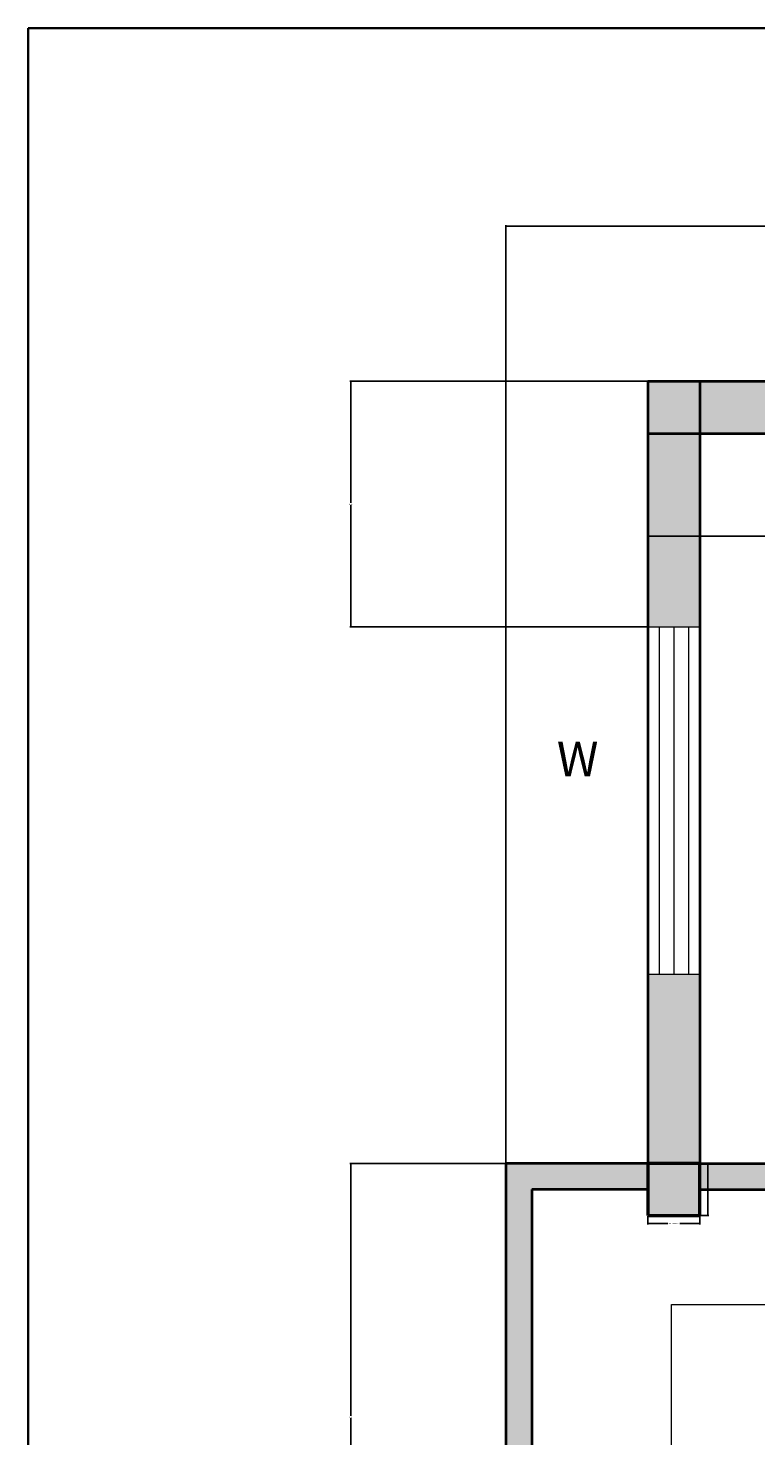
# Model space of a CAD drawing. Units: inches. Extents: x 25176543 to 25177243, y 80295576 to 80296086.
# Tile 2 of 11: x 25176543 to 25176668, y 80295843 to 80296086. Entities that reach past the tile are written whole.
import ezdxf

# ---------------------------------------------------------------- set-up
doc = ezdxf.new("R2010")
doc.units = ezdxf.units.IN
doc.header["$MEASUREMENT"] = 0
for name, color, linetype, lineweight in [('A-ANNO-DIMS', 2, 'Continuous', 18), ('A-ANNO-IDEN', 7, 'Continuous', 18), ('A-ANNO-SYMB', 7, 'Continuous', 18), ('A-ANNO-TTLB', 7, 'Continuous', 35), ('A-COLS', 7, 'Continuous', 50), ('A-COLS-PATT', 251, 'Continuous', 13), ('A-GLAZ', 4, 'Continuous', 18), ('A-WALL', 7, 'Continuous', 40), ('A-WALL-PATT', 146, 'Continuous', 13)]:
    doc.layers.add(name, color=color, linetype=linetype, lineweight=lineweight)
doc.styles.get("Standard").update_dxf_attribs({"font": 'arial.ttf'})
doc.dimstyles.get("Standard").update_dxf_attribs({"dimtxt": 0.18, "dimasz": 0.18, "dimexe": 0.18, "dimexo": 0.0625, "dimgap": 0.09, "dimtad": 0, "dimtih": 1, "dimtoh": 1, "dimdec": 4, "dimzin": 0, "dimdsep": 46, "dimtxsty": 'Standard', "dimcen": 0.09, "dimadec": 0, "dimazin": 0, "dimtfac": 1, "dimtdec": 4, "dimtofl": 0, "dimtmove": 0, "dimatfit": 3, "dimfxl": 1, "dimtolj": 1, "dimtzin": 0, "dimarcsym": 0})

# ---------------------------------------------------------------- blocks, each defined once
blk = doc.blocks.new('WIN-60IN')
for p, q in [((0, 9), (0, 0)), ((60, 9), (0, 9)), ((0, 9), (0, 4.5)), ((60, 0), (60, 9)), ((60, 7), (0, 7)), ((0, 4.5), (60, 4.5)), ((0, 2), (60, 2)), ((0, 0), (60, 0))]:
    blk.add_line(p, q)
blk = doc.blocks.new('COLUMN-9IN-SQ')
for p, q in [((9, 9), (0, 9)), ((0, 9), (0, 0)), ((9, 0), (9, 9)), ((0, 0), (9, 0))]:
    blk.add_line(p, q)
blk = doc.blocks.new('*D24')
at = {"layer": 'A-ANNO-DIMS', "color": 0, "lineweight": -2, "transparency": 16777216}
for p, q in [((25176649.8, 80295881.24), (25176649.8, 80295879.77)), ((25176649.98, 80295879.95), (25176653.26, 80295879.95)), ((25176658.62, 80295879.95), (25176655.34, 80295879.95)), ((25176658.8, 80295881.24), (25176658.8, 80295879.77))]:
    blk.add_line(p, q, dxfattribs=at)
at = {"layer": 'A-ANNO-DIMS', "color": 0, "transparency": 16777216}
for points in [[(25176649.98, 80295879.98), (25176649.98, 80295879.92), (25176649.8, 80295879.95)], [(25176658.62, 80295879.98), (25176658.62, 80295879.92), (25176658.8, 80295879.95)]]:
    blk.add_solid(points, dxfattribs=at)
at = {"layer": 'Defpoints', "color": 0, "transparency": 16777216}
for p in [(25176649.8, 80295881.3), (25176658.8, 80295881.3), (25176658.8, 80295879.95)]:
    blk.add_point(p, dxfattribs=at)
at = {"layer": 'A-ANNO-DIMS', "color": 0, "transparency": 16777216, "insert": (25176654.3, 80295879.95), "char_height": 0.18, "attachment_point": 5}
blk.add_mtext('\\A1;COLUMN 9 TYP.', dxfattribs=at)
blk = doc.blocks.new('*D25')
at = {"layer": 'A-ANNO-DIMS', "color": 0, "lineweight": -2, "transparency": 16777216}
for p, q in [((25176658.86, 80295890.3), (25176660.33, 80295890.3)), ((25176660.15, 80295890.12), (25176660.15, 80295885.98)), ((25176660.15, 80295881.48), (25176660.15, 80295885.62)), ((25176658.86, 80295881.3), (25176660.33, 80295881.3))]:
    blk.add_line(p, q, dxfattribs=at)
at = {"layer": 'A-ANNO-DIMS', "color": 0, "transparency": 16777216}
for points in [[(25176660.12, 80295890.12), (25176660.18, 80295890.12), (25176660.15, 80295890.3)], [(25176660.12, 80295881.48), (25176660.18, 80295881.48), (25176660.15, 80295881.3)]]:
    blk.add_solid(points, dxfattribs=at)
at = {"layer": 'Defpoints', "color": 0, "transparency": 16777216}
for p in [(25176658.8, 80295890.3), (25176660.15, 80295890.3), (25176658.8, 80295881.3)]:
    blk.add_point(p, dxfattribs=at)
at = {"layer": 'A-ANNO-DIMS', "color": 0, "transparency": 16777216, "insert": (25176660.15, 80295885.8), "char_height": 0.18, "attachment_point": 5}
blk.add_mtext('\\A1;9 TYP.', dxfattribs=at)
blk = doc.blocks.new('*D48')
at = {"layer": 'A-ANNO-DIMS', "color": 0, "lineweight": -2, "transparency": 16777216}
for p, q in [((25176625.3, 80295890.36), (25176625.3, 80296052.23)), ((25176625.48, 80296052.05), (25176875.16, 80296052.05)), ((25177125.62, 80296052.05), (25176875.95, 80296052.05)), ((25177125.8, 80296025.36), (25177125.8, 80296052.23))]:
    blk.add_line(p, q, dxfattribs=at)
at = {"layer": 'A-ANNO-DIMS', "color": 0, "transparency": 16777216}
for points in [[(25176625.48, 80296052.08), (25176625.48, 80296052.02), (25176625.3, 80296052.05)], [(25177125.62, 80296052.08), (25177125.62, 80296052.02), (25177125.8, 80296052.05)]]:
    blk.add_solid(points, dxfattribs=at)
at = {"layer": 'Defpoints', "color": 0, "transparency": 16777216}
for p in [(25177125.8, 80296052.05), (25177125.8, 80296025.3), (25176625.3, 80295890.3)]:
    blk.add_point(p, dxfattribs=at)
at = {"layer": 'A-ANNO-DIMS', "color": 0, "transparency": 16777216, "insert": (25176875.55, 80296052.05), "char_height": 0.18, "attachment_point": 5}
blk.add_mtext('\\A1;500.5', dxfattribs=at)
blk = doc.blocks.new('*D51')
at = {"layer": 'A-ANNO-DIMS', "color": 0, "lineweight": -2, "transparency": 16777216}
for p, q in [((25176625.24, 80295890.3), (25176598.37, 80295890.3)), ((25176598.55, 80295890.12), (25176598.55, 80295846.73)), ((25176598.55, 80295802.98), (25176598.55, 80295846.37)), ((25176625.24, 80295802.8), (25176598.37, 80295802.8))]:
    blk.add_line(p, q, dxfattribs=at)
at = {"layer": 'A-ANNO-DIMS', "color": 0, "transparency": 16777216}
for points in [[(25176598.52, 80295890.12), (25176598.58, 80295890.12), (25176598.55, 80295890.3)], [(25176598.52, 80295802.98), (25176598.58, 80295802.98), (25176598.55, 80295802.8)]]:
    blk.add_solid(points, dxfattribs=at)
at = {"layer": 'Defpoints', "color": 0, "transparency": 16777216}
for p in [(25176598.55, 80295890.3), (25176625.3, 80295890.3), (25176625.3, 80295802.8)]:
    blk.add_point(p, dxfattribs=at)
at = {"layer": 'A-ANNO-DIMS', "color": 0, "transparency": 16777216, "insert": (25176598.55, 80295846.55), "char_height": 0.18, "attachment_point": 5}
blk.add_mtext('\\A1;87.5', dxfattribs=at)
blk = doc.blocks.new('*D58')
at = {"layer": 'A-ANNO-DIMS', "color": 0, "lineweight": -2, "transparency": 16777216}
for p, q in [((25176649.74, 80296025.3), (25176598.37, 80296025.3)), ((25176598.55, 80296025.12), (25176598.55, 80296004.3)), ((25176598.55, 80295983.11), (25176598.55, 80296003.93)), ((25176649.74, 80295982.93), (25176598.37, 80295982.93))]:
    blk.add_line(p, q, dxfattribs=at)
at = {"layer": 'A-ANNO-DIMS', "color": 0, "transparency": 16777216}
for points in [[(25176598.52, 80296025.12), (25176598.58, 80296025.12), (25176598.55, 80296025.3)], [(25176598.52, 80295983.11), (25176598.58, 80295983.11), (25176598.55, 80295982.93)]]:
    blk.add_solid(points, dxfattribs=at)
at = {"layer": 'Defpoints', "color": 0, "transparency": 16777216}
for p in [(25176598.55, 80296025.3), (25176649.8, 80296025.3), (25176649.8, 80295982.93)]:
    blk.add_point(p, dxfattribs=at)
at = {"layer": 'A-ANNO-DIMS', "color": 0, "transparency": 16777216, "insert": (25176598.55, 80296004.11), "char_height": 0.18, "attachment_point": 5}
blk.add_mtext('\\A1;42.38', dxfattribs=at)
blk = doc.blocks.new('*D63')
at = {"layer": 'A-ANNO-DIMS', "color": 0, "lineweight": -2, "transparency": 16777216}
for p, q in [((25176649.8, 80296025.24), (25176649.8, 80295998.37)), ((25176695.19, 80296025.24), (25176695.19, 80295998.37)), ((25176649.98, 80295998.55), (25176672.1, 80295998.55)), ((25176695.01, 80295998.55), (25176672.89, 80295998.55))]:
    blk.add_line(p, q, dxfattribs=at)
at = {"layer": 'A-ANNO-DIMS', "color": 0, "transparency": 16777216}
for points in [[(25176649.98, 80295998.58), (25176649.98, 80295998.52), (25176649.8, 80295998.55)], [(25176695.01, 80295998.58), (25176695.01, 80295998.52), (25176695.19, 80295998.55)]]:
    blk.add_solid(points, dxfattribs=at)
at = {"layer": 'Defpoints', "color": 0, "transparency": 16777216}
for p in [(25176649.8, 80296025.3), (25176695.19, 80296025.3), (25176649.8, 80295998.55)]:
    blk.add_point(p, dxfattribs=at)
at = {"layer": 'A-ANNO-DIMS', "color": 0, "transparency": 16777216, "insert": (25176672.5, 80295998.55), "char_height": 0.18, "attachment_point": 5}
blk.add_mtext('\\A1;45.39', dxfattribs=at)

msp = doc.modelspace()

# ---------------------------------------------------------------- hatches: boundary and pattern name
at = {"layer": 'A-COLS-PATT'}
h = msp.add_hatch(color=256, dxfattribs=at)
h.dxf.hatch_style = 1
h.paths.add_polyline_path([(25176658.8016, 80296025.3022), (25176649.8016, 80296025.3022), (25176649.8016, 80296016.3022), (25176658.8016, 80296016.3022)])
h.paths.add_polyline_path([(25176819.3016, 80296025.3022), (25176810.3016, 80296025.3022), (25176810.3016, 80296016.3022), (25176819.3016, 80296016.3022)])
h.paths.add_polyline_path([(25176876.3016, 80296025.3022), (25176867.3016, 80296025.3022), (25176867.3016, 80296016.3022), (25176876.3016, 80296016.3022)])
h.paths.add_polyline_path([(25177013.3016, 80296025.3022), (25177004.3016, 80296025.3022), (25177004.3016, 80296016.3022), (25177013.3016, 80296016.3022)])
h.paths.add_polyline_path([(25176819.3016, 80295890.3022), (25176810.3016, 80295890.3022), (25176810.3016, 80295881.3022), (25176819.3016, 80295881.3022)])
h.paths.add_polyline_path([(25176658.8016, 80295890.3022), (25176649.8016, 80295890.3022), (25176649.8016, 80295881.3022), (25176658.8016, 80295881.3022)])
h.paths.add_polyline_path([(25177125.8016, 80296025.3022), (25177116.8016, 80296025.3022), (25177116.8016, 80296016.3022), (25177125.8016, 80296016.3022)])
h.paths.add_polyline_path([(25177125.8016, 80295848.3022), (25177116.8016, 80295848.3022), (25177116.8016, 80295839.3022), (25177125.8016, 80295839.3022)])
h.paths.add_polyline_path([(25177013.3016, 80295848.3022), (25177004.3016, 80295848.3022), (25177004.3016, 80295839.3022), (25177013.3016, 80295839.3022)])
h.paths.add_polyline_path([(25177125.8016, 80295676.8022), (25177116.8016, 80295676.8022), (25177116.8016, 80295667.8022), (25177125.8016, 80295667.8022)])
h.paths.add_polyline_path([(25177013.3016, 80295676.8022), (25177004.3016, 80295676.8022), (25177004.3016, 80295667.8022), (25177013.3016, 80295667.8022)])
h.paths.add_polyline_path([(25176842.3016, 80295676.8022), (25176833.3016, 80295676.8022), (25176833.3016, 80295667.8022), (25176842.3016, 80295667.8022)])
h.paths.add_polyline_path([(25176893.3016, 80295676.8022), (25176884.3016, 80295676.8022), (25176884.3016, 80295667.8022), (25176893.3016, 80295667.8022)])
h.paths.add_polyline_path([(25176842.3016, 80295807.3022), (25176833.3016, 80295807.3022), (25176833.3016, 80295798.3022), (25176842.3016, 80295798.3022)])
h.paths.add_polyline_path([(25176658.8016, 80295807.3022), (25176649.8016, 80295807.3022), (25176649.8016, 80295798.3022), (25176658.8016, 80295798.3022)])
h.paths.add_polyline_path([(25176658.8016, 80295676.8022), (25176649.8016, 80295676.8022), (25176649.8016, 80295667.8022), (25176658.8016, 80295667.8022)])
at = {"layer": 'A-WALL-PATT'}
h = msp.add_hatch(color=256, dxfattribs=at)
h.dxf.hatch_style = 1
h.paths.add_polyline_path([(25176695.189, 80296025.3022), (25176658.8016, 80296025.3022), (25176658.8016, 80296016.3022), (25176695.189, 80296016.3022)])
h.paths.add_polyline_path([(25176810.3016, 80296025.3022), (25176755.189, 80296025.3022), (25176755.189, 80296016.3022), (25176810.3016, 80296016.3022)])
h.paths.add_polyline_path([(25176819.3016, 80296016.3022), (25176814.8016, 80296016.3022), (25176814.8016, 80295965.3022), (25176819.3016, 80295965.3022)], flags=17)
h.paths.add_polyline_path([(25176828.0421, 80296025.3022), (25176819.3016, 80296025.3022), (25176819.3016, 80296016.3022), (25176828.0421, 80296016.3022)])
h.paths.add_polyline_path([(25176867.3016, 80296025.3022), (25176852.0421, 80296025.3022), (25176852.0421, 80296016.3022), (25176867.3016, 80296016.3022)])
h.paths.add_polyline_path([(25176885.1873, 80296025.3022), (25176876.3016, 80296025.3022), (25176876.3016, 80296016.3022), (25176885.1873, 80296016.3022)])
h.paths.add_polyline_path([(25176919.8016, 80296025.3022), (25176909.1873, 80296025.3022), (25176909.1873, 80296016.3022), (25176919.8016, 80296016.3022)])
h.paths.add_polyline_path([(25176924.3016, 80296016.3022), (25176919.8016, 80296016.3022), (25176919.8016, 80295890.3022), (25176904.8016, 80295890.3022), (25176904.8016, 80295885.8022), (25176967.3016, 80295885.8022), (25176967.3016, 80295890.3022), (25176924.3016, 80295890.3022)])
h.paths.add_polyline_path([(25176924.3016, 80296025.3022), (25176919.8016, 80296025.3022), (25176919.8016, 80296016.3022), (25176924.3016, 80296016.3022)])
h.paths.add_polyline_path([(25176938.7147, 80296025.3022), (25176924.3016, 80296025.3022), (25176924.3016, 80296016.3022), (25176938.7147, 80296016.3022)])
h.paths.add_polyline_path([(25176871.8016, 80296016.3022), (25176867.3016, 80296016.3022), (25176867.3016, 80295932.3022), (25176819.3016, 80295932.3022), (25176819.3016, 80295933.3022), (25176814.8016, 80295933.3022), (25176814.8016, 80295932.3022), (25176814.8016, 80295927.3022), (25176819.3016, 80295927.3022), (25176819.3016, 80295927.8022), (25176867.3016, 80295927.8022), (25176867.3016, 80295885.8022), (25176871.8016, 80295885.8022), (25176872.8016, 80295885.8022), (25176872.8016, 80295890.3022), (25176871.8016, 80295890.3022)])
h.paths.add_polyline_path([(25177004.3016, 80296025.3022), (25176986.7147, 80296025.3022), (25176986.7147, 80296016.3022), (25177004.3016, 80296016.3022)])
h.paths.add_polyline_path([(25177035.845, 80296025.3022), (25177013.3016, 80296025.3022), (25177013.3016, 80296016.3022), (25177035.845, 80296016.3022)])
h.paths.add_polyline_path([(25177008.8016, 80296016.3022), (25177004.3016, 80296016.3022), (25177004.3016, 80295890.3022), (25177003.3016, 80295890.3022), (25177003.3016, 80295885.8022), (25177004.3016, 80295885.8022), (25177004.3016, 80295885.3022), (25177008.8016, 80295885.3022)])
h.paths.add_polyline_path([(25177116.8016, 80296025.3022), (25177095.845, 80296025.3022), (25177095.845, 80296016.3022), (25177116.8016, 80296016.3022)])
h.paths.add_polyline_path([(25177125.8016, 80296016.3022), (25177116.8016, 80296016.3022), (25177116.8016, 80295971.1334), (25177121.3016, 80295971.1334), (25177125.8016, 80295971.1334)])
h.paths.add_polyline_path([(25177116.8016, 80295848.3022), (25177013.3016, 80295848.3022), (25177013.3016, 80295843.8022), (25177116.8016, 80295843.8022)])
h.paths.add_polyline_path([(25177125.8016, 80295911.1334), (25177116.8016, 80295911.1334), (25177116.8016, 80295848.3022), (25177125.8016, 80295848.3022)])
h.paths.add_polyline_path([(25177008.8016, 80295802.3022), (25177004.3016, 80295802.3022), (25177004.3016, 80295676.8022), (25177008.8016, 80295676.8022)])
h.paths.add_polyline_path([(25176658.8016, 80295705.5694), (25176649.8016, 80295705.5694), (25176649.8016, 80295676.8022), (25176658.8016, 80295676.8022)])
h.paths.add_polyline_path([(25176658.8016, 80295798.3022), (25176649.8016, 80295798.3022), (25176649.8016, 80295765.5694), (25176654.3016, 80295765.5694), (25176658.8016, 80295765.5694)])
h.paths.add_polyline_path([(25176833.3016, 80295807.3022), (25176658.8016, 80295807.3022), (25176658.8016, 80295802.8022), (25176833.3016, 80295802.8022)])
h.paths.add_polyline_path([(25176842.3016, 80295761.3022), (25176837.8016, 80295761.3022), (25176837.8016, 80295676.8022), (25176842.3016, 80295676.8022)])
h.paths.add_polyline_path([(25176649.8016, 80295807.3022), (25176629.8016, 80295807.3022), (25176629.8016, 80295885.8022), (25176649.8016, 80295885.8022), (25176649.8016, 80295890.3022), (25176625.3016, 80295890.3022), (25176625.3016, 80295802.8022), (25176649.8016, 80295802.8022)])
h.paths.add_polyline_path([(25176810.3016, 80295890.3022), (25176658.8016, 80295890.3022), (25176658.8016, 80295885.8022), (25176810.3016, 80295885.8022)])
h.paths.add_polyline_path([(25176658.8016, 80295922.9263), (25176649.8016, 80295922.9263), (25176649.8016, 80295890.3022), (25176658.8016, 80295890.3022)])
h.paths.add_polyline_path([(25176658.8016, 80296016.3022), (25176649.8016, 80296016.3022), (25176649.8016, 80295982.9263), (25176654.3016, 80295982.9263), (25176658.8016, 80295982.9263)])

# ---------------------------------------------------------------- linework, layer by layer
at = {"layer": 'A-ANNO-SYMB'}
for p, q in [((25176653.8935, 80295825.3022), (25176653.8935, 80295865.9686)), ((25176653.8935, 80295865.9686), (25176711.8016, 80295865.9686))]:
    msp.add_line(p, q, dxfattribs=at)
at = {"layer": 'A-ANNO-TTLB'}
msp.add_lwpolyline([(25176542.8973, 80296086.2335), (25177242.9194, 80296086.2335), (25177242.9194, 80295575.9501), (25176542.8973, 80295575.9501)], close=True, dxfattribs=at)
at = {"layer": 'A-WALL'}
for p, q in [((25176649.8016, 80296025.3022), (25177125.8016, 80296025.3022)), ((25176649.8016, 80296025.3022), (25176649.8016, 80295885.8022)), ((25176658.8016, 80296025.3022), (25176658.8016, 80295885.8022)), ((25176649.8016, 80296016.3022), (25177125.8016, 80296016.3022)), ((25176625.3016, 80295890.3022), (25176625.3016, 80295802.8022)), ((25176649.8016, 80295890.3022), (25176625.3016, 80295890.3022)), ((25176649.8016, 80295890.3022), (25176819.3016, 80295890.3022)), ((25176649.8016, 80295890.3022), (25176819.3016, 80295890.3022)), ((25176649.8016, 80295885.8022), (25176629.8016, 80295885.8022)), ((25176629.8016, 80295885.8022), (25176629.8016, 80295807.3022)), ((25176658.8016, 80295885.8022), (25176810.3016, 80295885.8022)), ((25176658.8016, 80295885.8022), (25176810.3016, 80295885.8022))]:
    msp.add_line(p, q, dxfattribs=at)

# ---------------------------------------------------------------- block references
at = {"layer": 'A-COLS'}
msp.add_blockref('COLUMN-9IN-SQ', (25176649.802, 80295881.302), dxfattribs=at)
at = {"layer": 'A-GLAZ', "extrusion": (0, 0, -1), "zscale": -1, "rotation": 270.0000000513552}
msp.add_blockref('WIN-60IN', (-25176658.8018, 80295982.9263), dxfattribs=at)

# ---------------------------------------------------------------- texts
at = {"layer": 'A-ANNO-IDEN', "insert": (25176634.1063, 80295963.1053), "char_height": 6, "attachment_point": 1}
msp.add_mtext_dynamic_manual_height_columns('W', width=24.139595, gutter_width=1, heights=[0], dxfattribs=at)

# ---------------------------------------------------------------- dimensions: what is measured, and where the dimension line sits
at = {"layer": 'A-ANNO-DIMS'}
dim = msp.add_linear_dim(base=(25177125.8016, 80296052.0522), p1=(25176625.3016, 80295890.3022), p2=(25177125.8016, 80296025.3022), dimstyle='Standard', override={"dimdec": 1, "dimlfac": 1, "dimrnd": 0, "dimzin": 0, "dimdsep": 46, "dimlunit": 2}, dxfattribs=at)
dim.commit()
dim.dimension.update_dxf_attribs({"geometry": '*D48', "text_midpoint": (25176875.5516, 80296052.0522)})
for base, p1, p2, angle, override, picture, middle in [((25176598.5516, 80296025.3022), (25176649.8016, 80295982.9263), (25176649.8016, 80296025.3022), 90, {"dimdec": 2, "dimlfac": 1, "dimrnd": 0, "dimzin": 0, "dimdsep": 46, "dimlunit": 2}, '*D58', (25176598.5516, 80296004.1142)), ((25176649.8016, 80295998.5522), (25176695.189, 80296025.3022), (25176649.8016, 80296025.3022), 180, {"dimdec": 2, "dimlfac": 1, "dimrnd": 0, "dimzin": 0, "dimdsep": 46, "dimlunit": 2}, '*D63', (25176672.4953, 80295998.5522)), ((25176598.5516, 80295890.3022), (25176625.3016, 80295802.8022), (25176625.3016, 80295890.3022), 90, {"dimdec": 1, "dimlfac": 1, "dimrnd": 0, "dimzin": 0, "dimdsep": 46, "dimlunit": 2}, '*D51', (25176598.5516, 80295846.5522))]:
    dim = msp.add_linear_dim(base=base, p1=p1, p2=p2, angle=angle, dimstyle='Standard', override=override, dxfattribs=at)
    dim.commit()
    dim.dimension.update_dxf_attribs({"geometry": picture, "text_midpoint": middle})
dim = msp.add_linear_dim(base=(25176660.1516, 80295890.3022), p1=(25176658.8016, 80295881.3022), p2=(25176658.8016, 80295890.3022), angle=90, text='<> TYP.', dimstyle='Standard', override={"dimdec": 0, "dimlfac": 1, "dimrnd": 0, "dimzin": 0, "dimdsep": 46, "dimlunit": 2}, dxfattribs=at)
dim.commit()
dim.dimension.update_dxf_attribs({"geometry": '*D25', "text_midpoint": (25176660.1516, 80295885.8022)})
dim = msp.add_linear_dim(base=(25176658.8016, 80295879.9522), p1=(25176649.8016, 80295881.3022), p2=(25176658.8016, 80295881.3022), text='COLUMN <> TYP.', dimstyle='Standard', override={"dimdec": 0, "dimlfac": 1, "dimrnd": 0, "dimzin": 0, "dimdsep": 46, "dimlunit": 2}, dxfattribs=at)
dim.commit()
dim.dimension.update_dxf_attribs({"geometry": '*D24', "text_midpoint": (25176654.3016, 80295879.9522)})

doc.saveas('drawing.dxf')
